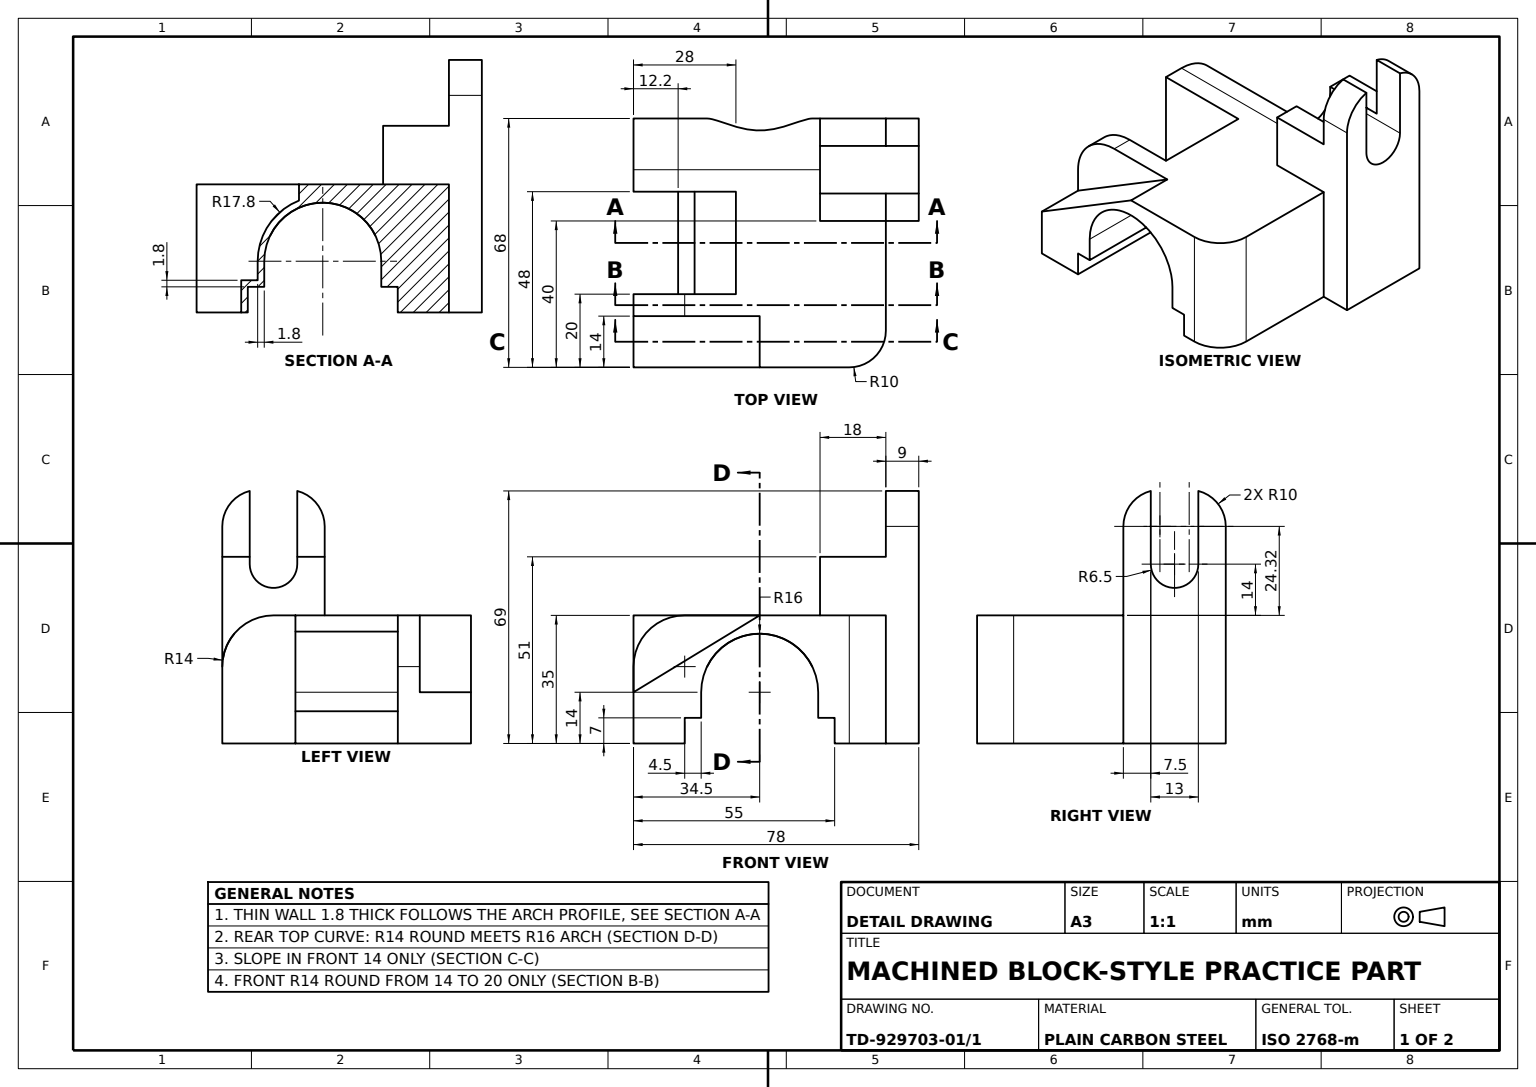
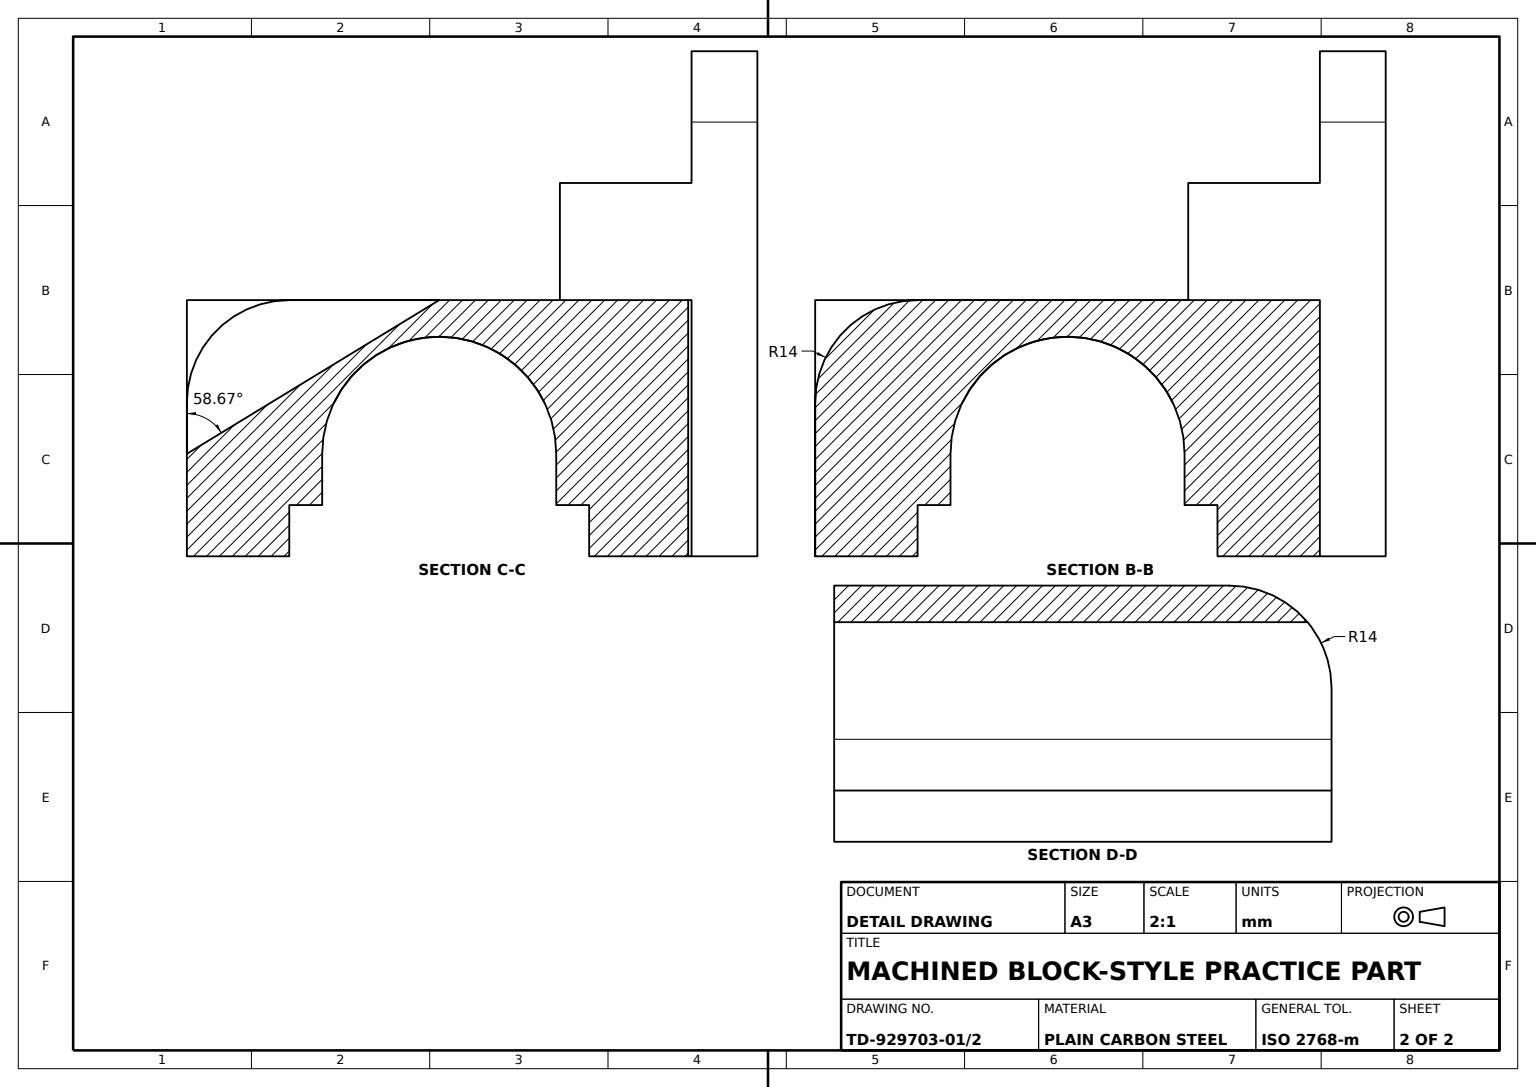
from build123d import *

# Parameters (mm, degrees)
BASE_BODY_20MM_DEPTH       = 20
BASE_START                 = -14
BASE_SLOT_CUT_DEPTH        = 14
THIN_START                 = -68
THIN_WALL_BOSS_1_8MM_DEPTH = 68
JOURNAL_BLOCK_BOSS_DEPTH   = 69
JOURNAL_START              = -69
JOURNAL_BORE_CUT_DEPTH     = 69
JOURNAL_RELIEF_CUT_DEPTH   = 69
CROSS_ARM_BOSS_DEPTH       = 9
UPRIGHT_LUG_SKETCH_W       = 28
UPRIGHT_LUG_SKETCH_H       = 41
UPRIGHT_LUG_BOSS_DEPTH     = 35
LUG_START                  = -69
LUG_SLOT_CUT_DEPTH         = 69
SIDE_START                 = 18
SIDE_RIB_BOSS_DEPTH        = 18
BASE_EDGE_FILLET_R10_R     = 10


with BuildPart() as part:
    # Base Profile Sketch → Base Body 20mm (new body)
    with BuildSketch(Plane(origin=(0, 0, 0), x_dir=(0, 0, -1), z_dir=(1, 0, 0))):
        with BuildLine():
            Line((20.5, 0), (20.5, 7))
            Line((20.5, 7), (16, 7))
            Line((16, 7), (16, 14))
            ThreePointArc((16, 14), (0, 30), (-16, 14))
            Line((-16, 14), (-16, 7))
            Line((-16, 7), (-20.5, 7))
            Line((-20.5, 7), (-20.5, 0))
            Line((-20.5, 0), (-34.5, 0))
            Line((-34.5, 0), (-34.5, 21))
            ThreePointArc((-34.5, 21), (-30.399494937, 30.899494937), (-20.5, 35))
            Line((-20.5, 35), (34.5, 35))
            Line((34.5, 35), (34.5, 0))
            Line((34.5, 0), (20.5, 0))
        make_face()
    extrude(amount=BASE_BODY_20MM_DEPTH)

    # Base Slot Sketch → Base Slot Cut (cut)
    with BuildSketch(Plane(origin=(20, 0, 0), x_dir=(0, 0, -1), z_dir=(1, 0, 0)).offset(BASE_START)):
        with BuildLine():
            Line((-34.5, 14), (0, 35))
            Line((0, 35), (-20.5, 35))
            ThreePointArc((-20.5, 35), (-30.399494937, 30.899494937), (-34.5, 21))
            Line((-34.5, 21), (-34.5, 14))
        make_face()
    extrude(amount=BASE_SLOT_CUT_DEPTH, mode=Mode.SUBTRACT)

    # Thin Wall Profile Sketch → Thin Wall Boss 1.8mm (add)
    with BuildSketch(Plane(origin=(20, 0, 0), x_dir=(0, 0, -1), z_dir=(1, 0, 0)).offset(THIN_START)):
        with BuildLine():
            Line((-16, 14), (-16, 7))
            Line((-16, 7), (-20.5, 7))
            Line((-20.5, 7), (-20.5, 0))
            Line((-20.5, 0), (-22.3, 0))
            Line((-22.3, 0), (-22.3, 8.8))
            Line((-22.3, 8.8), (-17.8, 8.8))
            Line((-17.8, 8.8), (-17.8, 14))
            ThreePointArc((-17.8, 14), (0, 31.8), (17.8, 14))
            Line((17.8, 14), (17.8, 8.8))
            Line((17.8, 8.8), (22.3, 8.8))
            Line((22.3, 8.8), (22.3, 0))
            Line((22.3, 0), (20.5, 0))
            Line((20.5, 0), (20.5, 7))
            Line((20.5, 7), (16, 7))
            Line((16, 7), (16, 14))
            ThreePointArc((16, 14), (0, 30), (-16, 14))
        make_face()
    extrude(amount=THIN_WALL_BOSS_1_8MM_DEPTH)

    # Journal Block Sketch → Journal Block Boss (add)
    with BuildSketch(Plane.XY.offset(34.5)):
        with BuildLine():
            Line((-48, 0), (-28, 0))
            Line((-28, 0), (-28, 35))
            Line((-28, 35), (-34, 35))
            ThreePointArc((-34, 35), (-43.899494937, 30.899494937), (-48, 21))
            Line((-48, 21), (-48, 0))
        make_face()
    extrude(amount=-JOURNAL_BLOCK_BOSS_DEPTH)

    # Journal Bore Sketch → Journal Bore Cut (cut)
    with BuildSketch(Plane(origin=(20, 0, 0), x_dir=(0, 0, -1), z_dir=(1, 0, 0)).offset(JOURNAL_START)):
        with BuildLine():
            Line((-16, 14), (-16, 7))
            Line((-16, 7), (-20.5, 7))
            Line((-20.5, 7), (-20.5, 0))
            Line((-20.5, 0), (20.5, 0))
            Line((20.5, 0), (20.5, 7))
            Line((20.5, 7), (16, 7))
            Line((16, 7), (16, 14))
            ThreePointArc((16, 14), (0, 30), (-16, 14))
        make_face()
    extrude(amount=JOURNAL_BORE_CUT_DEPTH, mode=Mode.SUBTRACT)

    # Journal Relief Sketch → Journal Relief Cut (cut)
    with BuildSketch(Plane.XY.offset(34.5)):
        with BuildLine():
            Line((-48, 21), (-48, 35))
            Line((-48, 35), (-34, 35))
            ThreePointArc((-34, 35), (-43.899494937, 30.899494937), (-48, 21))
        make_face()
    extrude(amount=-JOURNAL_RELIEF_CUT_DEPTH, mode=Mode.SUBTRACT)

    # Cross Arm Sketch → Cross Arm Boss (add)
    with BuildSketch(Plane(origin=(0, 0, -34.5), x_dir=(-1, 0, 0), z_dir=(0, 0, -1))):
        with BuildLine():
            Line((48, 21), (48, 35))
            Line((48, 35), (48, 59))
            Line((48, 59), (48, 59.317541634))
            ThreePointArc((48, 59.317541634), (45.90569415, 65.441265991), (40.5, 69))
            Line((40.5, 69), (40.5, 49))
            ThreePointArc((40.5, 49), (34, 42.5), (27.5, 49))
            Line((27.5, 49), (27.5, 69))
            ThreePointArc((27.5, 69), (22.09430585, 65.441265991), (20, 59.317541634))
            Line((20, 59.317541634), (20, 21))
            Line((20, 21), (20, 0))
            Line((20, 0), (48, 0))
            Line((48, 0), (48, 21))
        make_face()
    extrude(amount=CROSS_ARM_BOSS_DEPTH)

    # Upright Lug Sketch → Upright Lug Boss (add)
    with BuildSketch(Plane(origin=(0, 35, 0), x_dir=(1, 0, 0), z_dir=(0, 1, 0))):
        with Locations((-14, 14)):
            Rectangle(UPRIGHT_LUG_SKETCH_W, UPRIGHT_LUG_SKETCH_H)
    extrude(amount=-UPRIGHT_LUG_BOSS_DEPTH)

    # Lug Slot Sketch → Lug Slot Cut (cut)
    with BuildSketch(Plane(origin=(20, 0, 0), x_dir=(0, 0, -1), z_dir=(1, 0, 0)).offset(LUG_START)):
        with BuildLine():
            Line((-16, 14), (-16, 7))
            Line((-16, 7), (-20.5, 7))
            Line((-20.5, 7), (-20.5, 0))
            Line((-20.5, 0), (20.5, 0))
            Line((20.5, 0), (20.5, 7))
            Line((20.5, 7), (16, 7))
            Line((16, 7), (16, 14))
            ThreePointArc((16, 14), (0, 30), (-16, 14))
        make_face()
    extrude(amount=LUG_SLOT_CUT_DEPTH, mode=Mode.SUBTRACT)

    # Side Rib Sketch → Side Rib Boss (add)
    with BuildSketch(Plane.XY.offset(-34.5).offset(SIDE_START)):
        with BuildLine():
            Line((-20, 35), (-20, 51))
            Line((-20, 51), (-27.5, 51))
            Line((-27.5, 51), (-27.5, 49))
            ThreePointArc((-27.5, 49), (-34, 42.5), (-40.5, 49))
            Line((-40.5, 49), (-40.5, 51))
            Line((-40.5, 51), (-48, 51))
            Line((-48, 51), (-48, 21))
            ThreePointArc((-48, 21), (-43.899494937, 30.899494937), (-34, 35))
            Line((-34, 35), (-20, 35))
        make_face()
    extrude(amount=-SIDE_RIB_BOSS_DEPTH)

    # Base Edge Fillet R10
    base_edge_fillet_r10_edges = [part.edges().sort_by_distance(p)[0] for p in [
        (20, 17.5, -34.5),
    ]]
    fillet(base_edge_fillet_r10_edges, radius=BASE_EDGE_FILLET_R10_R)


solid = part.part
